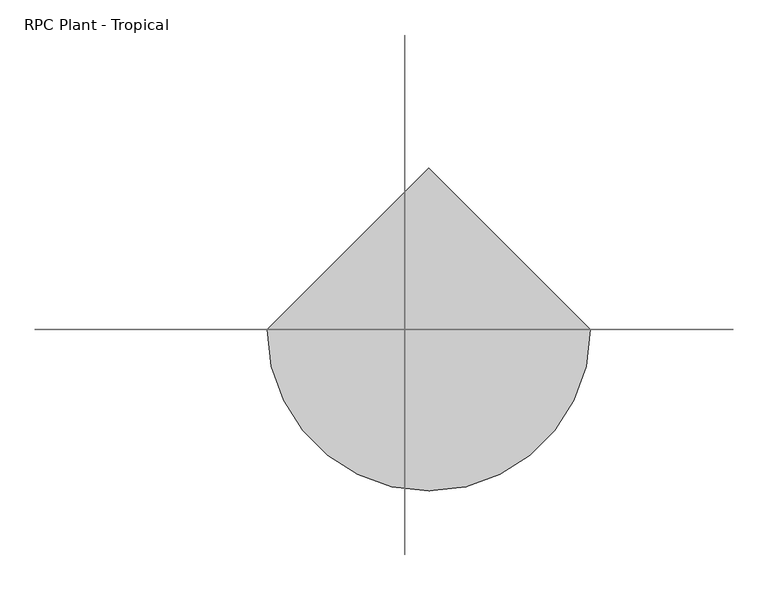
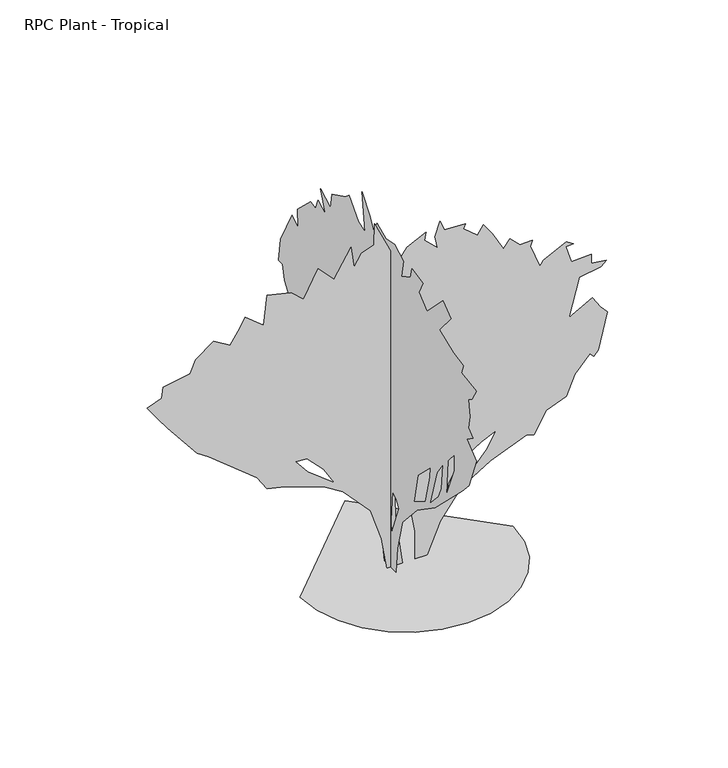
"""IFC4 building model written with IfcOpenShell, lengths in millimetres: geographic element geometry, RPC Plant - Tropical."""

from ifc_helpers import new_model, si_unit, origin, place, context, project, spatial, triangles, source, transform, mapped, element, save


def rpc_plant_tropical_6475341c(model_context):
    return source(origin(), model_context, "Body", "Tessellation", [
        triangles([(-396.3767504, 0.0, 8.22e-05), (-385.8992649, -90.8237077, 8.22e-05), (-356.0543206, -174.2306261, 8.22e-05), (-309.2370838, -247.8313661, 8.22e-05), (-247.8313661, -309.2370838, 8.22e-05), (-174.2306261, -356.0543206, 8.22e-05), (-90.8237077, -385.8992649, 8.22e-05), (1.73e-05, -396.3767504, 8.22e-05), (90.8237077, -385.8992649, 8.22e-05), (174.2306261, -356.0543206, 8.22e-05), (247.8313661, -309.2370838, 8.22e-05), (309.2370838, -247.8313661, 8.22e-05), (356.0543206, -174.2306261, 8.22e-05), (385.8992649, -90.8237077, 8.22e-05), (396.3767504, 3.47e-05, 8.22e-05), (-5.2e-05, 396.3767504, 8.22e-05), (-59.3577095, -35.0059915, 9.26e-05), (-59.3577095, -44.8705806, 101.5460546), (-59.3577095, -75.4742449, 222.0478563), (-59.3577095, -168.9964434, 326.3007588), (-59.3577095, -285.8741748, 405.6706235), (-59.3579639, -459.2340692, 576.3228888), (-59.3579639, -503.9253456, 625.6344137), (-59.3579639, -553.1479589, 751.1941189), (-59.3579639, -491.6190474, 799.7715317), (-59.3579639, -530.478485, 828.915465), (-59.3579639, -501.3320083, 851.5849388), (-59.3579639, -511.0474763, 900.1598808), (-59.3579639, -501.3320083, 961.688756), (-59.3579639, -524.0014821, 977.8812269), (-59.3579639, -553.1479589, 1026.4561689), (-59.3579639, -455.9955677, 1039.4101748), (-59.3579639, -469.4956884, 1077.0376745), (-59.3579639, -404.1821606, 1087.9850441), (-59.3579639, -313.5068087, 1123.6085238), (-59.3579639, -387.9896896, 1211.0454105), (-59.3579639, -336.1762825, 1249.9048119), (-59.3579639, -235.7859349, 1149.5164627), (-59.3579639, -183.9712561, 1191.6144018), (-59.3579639, -209.8784683, 1243.4278816), (-59.3579639, -138.9198272, 1256.3183739), (-59.3579639, -128.9188388, 1217.5224134), (-59.3579639, -70.6279291, 1185.1373989), (-59.3579639, -83.5816624, 1253.143277), (-59.3579639, -25.4436618, 1284.1769932), (-59.3579639, 29.761912, 1272.5743584), (-59.3579639, 86.0073592, 1299.3586246), (-59.3579639, 110.7212849, 1256.3817421), (-59.3579639, 133.3899957, 1298.4822247), (-59.3579639, 185.2039207, 1363.2496376), (-59.3577095, 165.7739475, 1217.5224134), (-59.3577095, 207.8728858, 1230.4738758), (-59.3577095, 266.3644464, 1299.9199276), (-59.3577095, 292.0717617, 1279.0512886), (-59.3577095, 376.2676217, 1236.950806), (-59.3577095, 385.9830897, 1178.660396), (-59.3577095, 450.7505027, 1214.2838757), (-59.3577095, 418.3680679, 1133.3239918), (-59.3577095, 466.9429736, 1159.22946), (-59.3577095, 484.2835213, 1117.1086298), (-59.3577095, 515.5204227, 1123.6085238), (-59.3577095, 599.7162646, 1042.6486399), (-59.3577095, 596.4777632, 974.6427618), (-59.3577095, 635.3397079, 997.3122356), (-59.3577095, 709.8225889, 858.0619417), (-59.3577095, 722.7765947, 767.3865898), (-59.3577095, 696.8686558, 767.3865898), (-59.3577095, 683.91465, 712.3346449), (-59.3577095, 619.147237, 621.659293), (-59.3577095, 586.7622588, 628.1362959), (-59.3577095, 577.0493342, 595.7513177), (-59.3577095, 544.664356, 589.2743148), (-59.3577095, 512.2819213, 514.7914338), (-59.3577095, 453.9890041, 501.8400078), (-59.3577095, 473.4199765, 479.1705339), (-59.3577095, 438.083507, 433.2245012), (-59.3577095, 424.8450708, 430.5955919), (-59.3577095, 359.671251, 388.3935531), (-59.3577095, 230.5626891, 332.9860339), (-59.3577095, 112.6590482, 224.7923109), (-59.3577095, 55.1474106, 87.2636415), (-59.3577095, 39.476642, 8.38e-05), (-59.3577095, -5.8605105, 135.9018064), (-59.3577095, -2.7896791, 186.1833303), (-59.3577095, -12.337225, 304.2967785), (-59.3577095, -38.2442317, 288.1068329), (-59.3577095, -54.4362076, 262.1988576), (-59.3577095, -151.5875587, 349.6357444), (-59.3577095, -177.4947618, 469.4550296), (-59.3577095, -258.4549001, 547.176412), (-59.3577095, -255.2163986, 508.3169744), (-59.3577095, -226.0704487, 394.9721486), (-59.3577095, -255.2163986, 404.687653), (-59.3577095, -297.3143196, 550.4149135), (-59.3577095, -337.517407, 606.5056758), (-59.3577095, -326.4607781, 505.0785092), (-59.3577095, -307.0298058, 462.9780267), (-59.3577095, -358.8432129, 501.8400078), (-59.3579639, -368.5587173, 641.0903017), (-59.3579639, -410.6591635, 689.6651711), (-59.3579639, -410.6591635, 628.1362959), (-59.3577095, 198.157654, 356.112711), (-59.3577095, 261.769596, 391.7057055), (-59.3577095, 324.4541782, 475.9320325), (-59.3577095, 282.3562755, 469.4550296), (-59.3577095, 253.2100531, 430.5955919), (-267.2940953, 2.61e-05, 404.687653), (-308.6096875, 2.21e-05, 471.3142911), (-370.9208914, 1.84e-05, 534.2224425), (-413.0213739, 1.82e-05, 537.4609076), (-368.4215527, 2.15e-05, 482.1804156), (30.6369404, 5.02e-05, 0.0), (31.1304627, 4.38e-05, 108.1619844), (9.0696959, 3.61e-05, 237.4841779), (-47.0839311, 3.05e-05, 330.2047357), (-39.4309189, 4.01e-05, 170.4041154), (-14.7000316, 5.02e-05, 0.0), (-72.990889, 5.02e-05, 0.0), (-92.9872747, 4.29e-05, 122.5858678), (-134.4006626, 3.55e-05, 247.1552083), (-236.0793036, 2.88e-05, 358.7517941), (-302.2063538, 2.64e-05, 398.8659516), (-451.8807753, 2.32e-05, 453.2625587), (-519.8892331, 2.22e-05, 469.4550296), (-555.510133, 1.89e-05, 524.5069382), (-736.858366, 1.03e-05, 670.234235), (-778.9587759, 8.5e-06, 699.3807117), (-889.0625931, 4e-07, 835.3924679), (-924.6860727, -2.5e-06, 883.9674099), (-965.6003632, -6e-06, 942.4685629), (-911.7320669, -7.1e-06, 961.688756), (-905.255064, -9.6e-06, 1003.7892385), (-804.8642441, -1.06e-05, 1019.979166), (-785.4357788, -1.35e-05, 1068.5565788), (-717.4299007, -1.64e-05, 1117.1315208), (-655.8984821, -1.43e-05, 1081.5105846), (-620.2775459, -1.75e-05, 1136.5625296), (-600.8465735, -1.97e-05, 1172.1833931), (-532.8406591, -1.64e-05, 1117.1315208), (-519.8892331, -2.31e-05, 1230.4738758), (-429.2138449, -2.18e-05, 1207.8068727), (-383.8748972, -1.93e-05, 1165.7064629), (-328.8229886, -2.53e-05, 1266.0972828), (-270.5325967, -2.16e-05, 1204.5684076), (-205.7644389, -2.78e-05, 1308.1951492), (-196.0496976, -2.29e-05, 1227.2378815), (-167.6639666, -2.55e-05, 1270.8241745), (-121.5665623, -2.66e-05, 1288.7668293), (-119.7654549, -3.15e-05, 1371.5986919), (-34.1304544, -2.06e-05, 1188.3759367), (2.3015577, -2.34e-05, 1235.4267712), (72.7363851, -2.54e-05, 1269.3357479), (66.2596456, -2.37e-05, 1240.1892712), (114.8353143, -2.1e-05, 1194.8529396), (105.1200825, -2.37e-05, 1240.1892712), (124.5505553, -2.7e-05, 1295.2437595), (140.7425266, -2.47e-05, 1256.3817421), (218.4636638, -2.45e-05, 1253.143277), (211.1367854, -2.35e-05, 1235.7950626), (263.8015941, -2.08e-05, 1191.6144018), (286.4685245, -2.27e-05, 1223.9994164), (318.8535027, -2e-05, 1178.660396), (360.9514054, -1.56e-05, 1104.177515), (385.0814006, -1.75e-05, 1135.7446289), (422.4828604, -1.52e-05, 1097.7005121), (467.8192646, -1.54e-05, 1100.9390499), (461.3422617, -1.41e-05, 1078.2721195), (496.9657413, -8.7e-06, 987.5967676), (509.9172037, -9.8e-06, 1007.0277037), (594.1155527, -1.23e-05, 1049.1256428), (620.0235643, -1.14e-05, 1032.9331718), (593.290058, -1.13e-05, 1031.1069025), (613.5465614, -7.3e-06, 964.9272211), (688.0294424, -7.5e-06, 968.1657589), (688.0294424, -5.4e-06, 932.5448227), (743.0813147, -5e-06, 926.0678198), (723.6503786, -3.8e-06, 906.6368837), (642.6904947, -3.1e-06, 893.6828779), (603.8310571, 5.6e-06, 747.9555811), (691.2679075, 2.7e-06, 796.5330666), (720.4118408, 5.4e-06, 751.1941189), (746.3198524, 7.2e-06, 722.0501856), (713.9348379, 1.55e-05, 582.7973482), (697.7449104, 1.66e-05, 563.3688829), (681.5524395, 1.57e-05, 579.5613902), (626.5005672, 1.93e-05, 518.0299353), (594.1155527, 2.38e-05, 443.5470543), (519.6326717, 2.55e-05, 414.403121), (474.2962675, 3.03e-05, 333.4432371), (448.3882922, 2.98e-05, 343.1587415), (311.7719945, 3.3e-05, 288.0331637), (205.1723602, 3.7e-05, 221.2502851), (125.3034072, 4.32e-05, 117.1220752), (75.9746277, 5.02e-05, 0.0), (30.6369404, 3.34e-05, 281.62983), (43.5909303, 2.72e-05, 385.2566442), (7.9686832, 2.28e-05, 459.7395252), (-30.8919575, 2.45e-05, 430.5955919), (-38.6976243, 2.72e-05, 386.112624), (-2.6646859, 3.14e-05, 315.8842435), (150.4575132, 3.75e-05, 213.6229345), (215.0437962, 3.57e-05, 242.9182394), (296.5269221, 3.01e-05, 337.5199505), (331.8074721, 2.65e-05, 398.2106501), (278.0814637, 2.79e-05, 375.0661689), (195.3344433, 3.11e-05, 320.3901821), (154.7673882, 3.52e-05, 251.8887493)], [[15, 16, 1], [14, 15, 1], [14, 1, 2], [13, 14, 2], [13, 2, 3], [13, 3, 4], [12, 13, 4], [11, 12, 4], [11, 4, 5], [11, 5, 6], [11, 6, 7], [11, 7, 8], [11, 8, 9], [11, 9, 10], [93, 90, 91], [93, 91, 92], [90, 93, 94], [95, 98, 99], [83, 17, 18], [98, 95, 96], [49, 50, 51], [56, 57, 58], [88, 85, 86], [48, 49, 51], [102, 84, 85], [83, 18, 19], [87, 83, 19], [30, 31, 32], [87, 19, 20], [39, 40, 41], [39, 41, 42], [25, 26, 27], [29, 30, 32], [82, 17, 83], [81, 82, 83], [80, 81, 83], [80, 83, 84], [80, 84, 102], [79, 80, 102], [79, 102, 103], [78, 79, 103], [78, 103, 104], [77, 78, 104], [32, 33, 34], [65, 66, 67], [58, 59, 60], [35, 36, 37], [35, 37, 38], [88, 86, 87], [88, 87, 20], [92, 88, 20], [92, 20, 21], [93, 92, 21], [97, 93, 21], [97, 21, 22], [63, 64, 65], [52, 53, 54], [46, 47, 48], [74, 75, 76], [23, 24, 25], [43, 44, 45], [43, 45, 46], [98, 96, 97], [98, 97, 22], [101, 98, 22], [101, 22, 23], [101, 23, 25], [100, 101, 25], [68, 69, 70], [74, 76, 77], [74, 77, 104], [70, 71, 72], [85, 88, 89], [102, 85, 89], [106, 102, 89], [105, 106, 89], [52, 54, 55], [52, 55, 56], [60, 61, 62], [60, 62, 63], [39, 42, 43], [72, 73, 74], [43, 46, 48], [43, 48, 51], [63, 65, 67], [90, 94, 95], [105, 89, 90], [38, 39, 43], [63, 67, 68], [63, 68, 70], [63, 70, 72], [60, 63, 72], [58, 60, 72], [58, 72, 74], [58, 74, 104], [58, 104, 105], [58, 105, 90], [56, 58, 90], [52, 56, 90], [51, 52, 90], [43, 51, 90], [38, 43, 90], [38, 90, 95], [38, 95, 99], [38, 99, 100], [35, 38, 100], [35, 100, 25], [35, 25, 27], [34, 35, 27], [32, 34, 27], [29, 32, 27], [28, 29, 27], [196, 112, 113], [196, 197, 201], [195, 196, 113], [195, 113, 114], [148, 149, 150], [112, 196, 201], [170, 171, 172], [207, 201, 197], [144, 145, 146], [155, 156, 157], [175, 176, 177], [175, 177, 178], [151, 152, 153], [194, 112, 201], [193, 194, 201], [192, 193, 201], [192, 201, 202], [191, 192, 202], [191, 202, 203], [195, 114, 115], [200, 195, 115], [199, 200, 115], [169, 170, 172], [206, 207, 197], [157, 158, 159], [165, 166, 167], [160, 161, 162], [142, 143, 144], [129, 130, 131], [116, 117, 118], [116, 118, 119], [116, 119, 120], [115, 116, 120], [107, 115, 120], [107, 120, 121], [107, 121, 122], [111, 107, 122], [111, 122, 123], [110, 111, 123], [137, 138, 139], [199, 115, 107], [163, 164, 165], [139, 140, 141], [183, 184, 185], [190, 191, 203], [190, 203, 204], [173, 174, 175], [173, 175, 178], [169, 172, 173], [179, 180, 181], [198, 199, 107], [139, 141, 142], [188, 189, 190], [110, 123, 124], [110, 124, 125], [168, 169, 173], [154, 155, 157], [154, 157, 159], [131, 132, 133], [182, 183, 185], [188, 190, 204], [147, 148, 150], [146, 147, 150], [205, 206, 197], [136, 137, 139], [181, 182, 185], [179, 181, 185], [179, 185, 186], [134, 135, 136], [198, 107, 108], [154, 159, 160], [133, 134, 136], [168, 173, 178], [168, 178, 179], [129, 131, 133], [128, 129, 133], [127, 128, 133], [127, 133, 136], [126, 127, 136], [126, 136, 139], [125, 126, 139], [110, 125, 139], [110, 139, 142], [109, 110, 142], [109, 142, 144], [109, 144, 146], [109, 146, 150], [108, 109, 150], [198, 108, 150], [197, 198, 150], [205, 197, 150], [204, 205, 150], [188, 204, 150], [187, 188, 150], [186, 187, 150], [179, 186, 150], [168, 179, 150], [167, 168, 150], [150, 151, 153], [150, 153, 154], [160, 162, 163], [154, 160, 163], [150, 154, 163], [167, 150, 163], [167, 163, 165]], closed=False),
    ])


if __name__ == "__main__":
    model = new_model("IFC4")
    model_context = context("Model", 3, world=origin())
    ifc_project = project(units=[si_unit("LENGTHUNIT", "METRE", prefix="MILLI")], contexts=[model_context])
    site = spatial("IfcSite", under=ifc_project)
    building = spatial("IfcBuilding", under=site)
    placement = place(None, origin())
    rpc_plant_tropical_shape = rpc_plant_tropical_6475341c(model_context)
    element("IfcGeographicElement", 1, ObjectType="RPC Plant - Tropical", at=placement, inside=building, context=model_context, shape_type="MappedRepresentation", body=[
        mapped(rpc_plant_tropical_shape, transform((0.0, 0.0, 0.0), x_axis=(1.0, 0.0, 0.0), y_axis=(0.0, 1.0, 0.0), z_axis=(0.0, 0.0, 1.0))),
    ])
    save(model, "model.ifc")

# Revit data of these elements
# Type "RPC Plant - Tropical"
#   built-in parameter 1005198 = "{2, 15},{39, RPC-16-G3GK-N2Q0-PN0G-6000-ST1L-LVER-AU},{1, 0},{1, 0},{2, 35},{1, 8},{5, Color},{1, 0},{1, 0},{3, 0.8},{3, 0.8},{3, 0.8},{1, 8},{7, BBoxMin},{1, 0},{1, 0},{1, 0},{1, 0},{1, 0},{1, 8},{7, BBoxMax},{1, 0},{1, 0},{1, 0},{1, 0},{1, 0},{2, 11},{9, RPCTypeId},{1, 0},{1, 0},{39, RPC-16-G3GK-N2Q0-PN0G-6000-ST1L-LVER-AU},{1, 6},{14, RPCPlantHeight},{1, 0},{1, 0},{3, 4.5},{2, 11},{7, keyword},{1, 0},{1, 0},{80, :Geometry:RPC:Honey Myrtle:honey myrtle:melaleuca spathulata:tropical:austrailia},{2, 11},{8, category},{1, 0},{1, 0},{17, :Shrubs [General]},{2, 11},{12, LocalizedUID},{1, 0},{1, 0},{12, Honey Myrtle},{2, 14},{6, Height},{1, 0},{1, 0},{3, 4.5},{1, 2},{16, Cast Reflections},{1, 0},{1, 0},{1, 0},{1, 2},{12, Cast Shadows},{1, 0},{1, 0},{1, 1},{1, 2},{9, Lock View},{1, 0},{1, 0},{1, 0},{1, 4},{5, ViewC},{1, 0},{1, 0},{1, 0},{2, 11},{20, AdvancedUIDefinition},{1, 0},{1, 0},{0, },{2, 11},{10, AssetLibID},{1, 0},{1, 0},{36, 4D3F6E72-3F99-4203-98E9-AF80B3C7A7A4},{2, 11},{10, BaseSchema},{1, 0},{1, 0},{9, RPCSchema},{2, 11},{12, ExchangeGUID},{1, 0},{1, 0},{0, },{1, 2},{6, Hidden},{1, 0},{1, 0},{1, 0},{1, 4},{11, RPCCategory},{1, 0},{1, 0},{1, 0},{2, 11},{8, RPCImage},{1, 0},{1, 0},{0, },{1, 4},{13, SchemaVersion},{1, 0},{1, 0},{1, 4},{2, 11},{12, UIDefinition},{1, 0},{1, 0},{0, },{2, 11},{6, UIName},{1, 0},{1, 0},{39, RPC-16-G3GK-N2Q0-PN0G-6000-ST1L-LVER-AU},{2, 11},{11, VersionGUID},{1, 0},{1, 0},{9, RPCSchema},{2, 11},{9, assettype},{1, 0},{1, 0},{11, RPCGeometry},{2, 11},{11, description},{1, 0},{1, 0},{0, },{2, 11},{9, localname},{1, 0},{1, 0},{3, RPC},{2, 11},{9, localtype},{1, 0},{1, 0},{3, RPC},{1, 4},{8, revision},{1, 0},{1, 0},{1, 1},{2, 11},{9, thumbnail},{1, 0},{1, 0},{0, },{1, 4},{7, version},{1, 0},{1, 0},{1, 1},{1, 2},{20, RPC_Cast Reflections},{1, 0},{1, 0},{1, 1},{1, 2},{16, RPC_Cast Shadows},{1, 0},{1, 0},{1, 1},{1, 2},{13, RPC_Lock View},{1, 0},{1, 0},{1, 0},{1, 4},{9, RPC_ViewC},{1, 0},{1, 0},{1, 0},{21, assetlibrary_base.fbx},{1, 5},"
#   built-in parameter 1005195 = "RPC-16-G3GK-N2Q0-PN0G-6000-ST1L-LVER-AU"
#   Assembly Code = "G2050500"
#   Height = 4' - 6"
#   Default Elevation = 0
